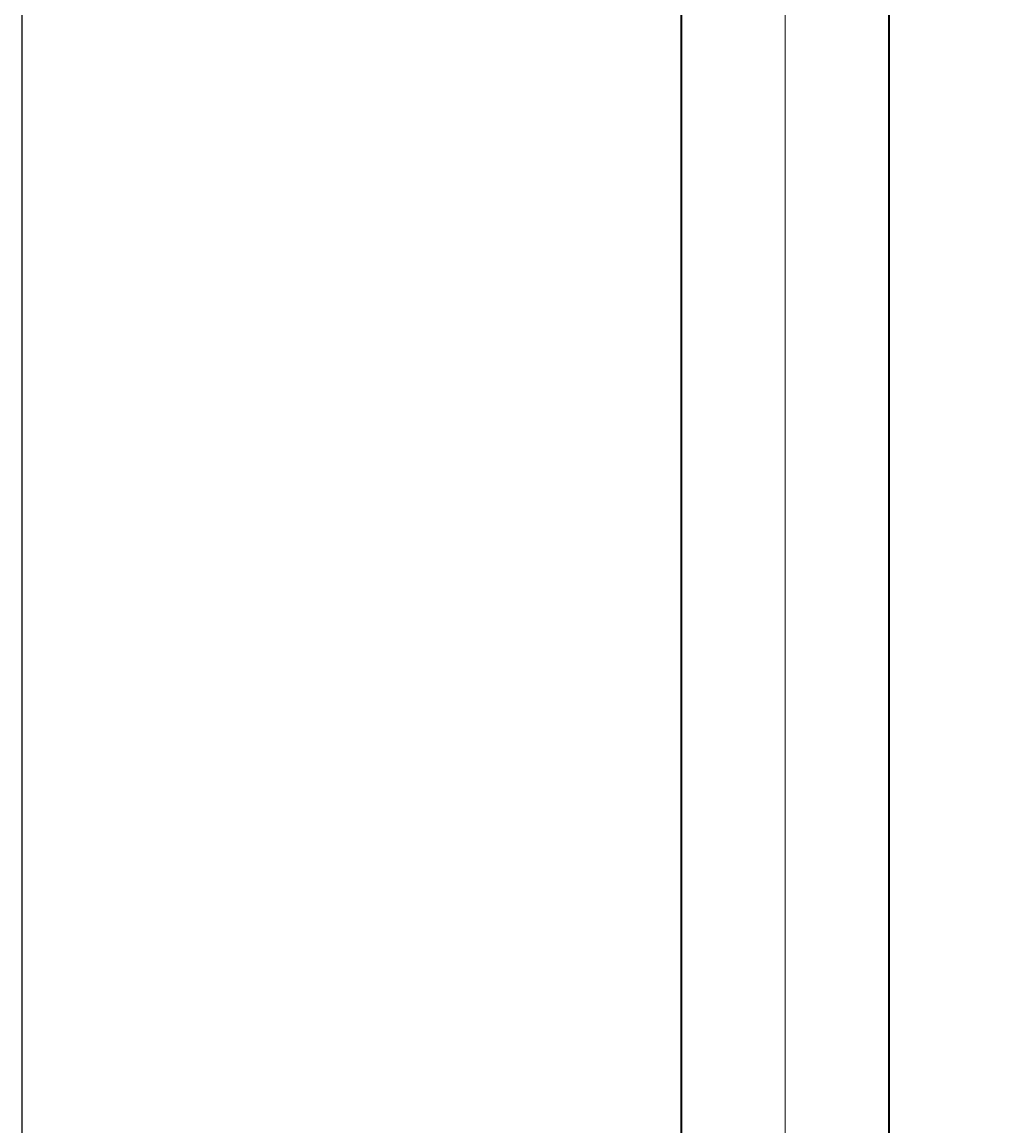
# Model space of a CAD drawing. Units: inches. Extents: x 1962 to 2771, y 1245 to 2660.
# Tile 44 of 114: x 2072 to 2093, y 2098 to 2122. Entities that reach past the tile are written whole.
import ezdxf

# ---------------------------------------------------------------- set-up
doc = ezdxf.new("R2010")
doc.units = ezdxf.units.IN
for name, color, linetype, lineweight in [('A-ANNO-DIMS', 2, 'Continuous', 18), ('A-GLAZ', 4, 'Continuous', 18), ('A-WALL', 7, 'Continuous', 35)]:
    doc.layers.add(name, color=color, linetype=linetype, lineweight=lineweight)
doc.styles.get("Standard").update_dxf_attribs({"font": 'arial.ttf'})
doc.dimstyles.get("Standard").update_dxf_attribs({"dimtxt": 0.18, "dimasz": 0.18, "dimexe": 0.18, "dimexo": 0.0625, "dimgap": 0.09, "dimtad": 0, "dimtih": 1, "dimtoh": 1, "dimdec": 4, "dimzin": 0, "dimdsep": 46, "dimtxsty": 'Standard', "dimcen": 0.09, "dimadec": 0, "dimazin": 0, "dimtfac": 1, "dimtdec": 4, "dimtofl": 0, "dimtmove": 0, "dimatfit": 3, "dimfxl": 1, "dimtolj": 1, "dimtzin": 0, "dimarcsym": 0})

# ---------------------------------------------------------------- blocks, each defined once
blk = doc.blocks.new('WIN-60IN-A')
blk.add_line((2.25, 60), (2.25, 0))
blk = doc.blocks.new('*D40')
at = {"layer": 'A-ANNO-DIMS', "color": 0, "lineweight": -2, "transparency": 16777216}
for p, q in [((2072.02, 2033.906), (2072.02, 2583.474)), ((2072.2, 2583.294), (2366.02, 2583.294)), ((2660.627, 2583.294), (2366.808, 2583.294)), ((2660.807, 2524.406), (2660.807, 2583.474))]:
    blk.add_line(p, q, dxfattribs=at)
at = {"layer": 'A-ANNO-DIMS', "color": 0, "transparency": 16777216}
for points in [[(2072.2, 2583.324), (2072.2, 2583.264), (2072.02, 2583.294)], [(2660.627, 2583.324), (2660.627, 2583.264), (2660.807, 2583.294)]]:
    blk.add_solid(points, dxfattribs=at)
at = {"layer": 'Defpoints', "color": 0, "transparency": 16777216}
for p in [(2660.807, 2583.294), (2660.807, 2524.344), (2072.02, 2033.844)]:
    blk.add_point(p, dxfattribs=at)
at = {"layer": 'A-ANNO-DIMS', "color": 0, "transparency": 16777216, "insert": (2366.414, 2583.294), "char_height": 0.18, "attachment_point": 5}
blk.add_mtext('\\A1;588.8', dxfattribs=at)
blk = doc.blocks.new('*D43')
at = {"layer": 'A-ANNO-DIMS', "color": 0, "lineweight": -2, "transparency": 16777216}
for p, q in [((2086.245, 2524.344), (2012.89, 2524.344)), ((2013.07, 2524.164), (2013.07, 2279.276)), ((2013.07, 2034.024), (2013.07, 2278.912)), ((2071.958, 2033.844), (2012.89, 2033.844))]:
    blk.add_line(p, q, dxfattribs=at)
at = {"layer": 'A-ANNO-DIMS', "color": 0, "transparency": 16777216}
for points in [[(2013.04, 2524.164), (2013.1, 2524.164), (2013.07, 2524.344)], [(2013.04, 2034.024), (2013.1, 2034.024), (2013.07, 2033.844)]]:
    blk.add_solid(points, dxfattribs=at)
at = {"layer": 'Defpoints', "color": 0, "transparency": 16777216}
for p in [(2086.307, 2524.344), (2013.07, 2033.844), (2072.02, 2033.844)]:
    blk.add_point(p, dxfattribs=at)
at = {"layer": 'A-ANNO-DIMS', "color": 0, "transparency": 16777216, "insert": (2013.07, 2279.094), "char_height": 0.18, "attachment_point": 5}
blk.add_mtext('\\A1;490.5', dxfattribs=at)

msp = doc.modelspace()

# ---------------------------------------------------------------- linework, layer by layer
at = {"layer": 'A-WALL'}
for p, q in [((2086.3074, 2471.8437), (2086.3074, 2033.8437)), ((2090.8074, 2177.8437), (2090.8074, 2033.8437))]:
    msp.add_line(p, q, dxfattribs=at)

# ---------------------------------------------------------------- block references
at = {"layer": 'A-GLAZ'}
msp.add_blockref('WIN-60IN-A', (2086.3074, 2080.0389), dxfattribs=at)

# ---------------------------------------------------------------- dimensions: what is measured, and where the dimension line sits
at = {"layer": 'A-ANNO-DIMS'}
dim = msp.add_linear_dim(base=(2660.8074, 2583.2937), p1=(2072.0204, 2033.8437), p2=(2660.8074, 2524.3437), dimstyle='Standard', override={"dimdec": 1, "dimlfac": 1, "dimrnd": 0, "dimzin": 0, "dimdsep": 46, "dimlunit": 2}, dxfattribs=at)
dim.commit()
dim.dimension.update_dxf_attribs({"geometry": '*D40', "text_midpoint": (2366.4139, 2583.2937)})
dim = msp.add_linear_dim(base=(2013.0704, 2033.8437), p1=(2086.3074, 2524.3437), p2=(2072.0204, 2033.8437), angle=90, dimstyle='Standard', override={"dimdec": 1, "dimlfac": 1, "dimrnd": 0, "dimzin": 0, "dimdsep": 46, "dimlunit": 2}, dxfattribs=at)
dim.commit()
dim.dimension.update_dxf_attribs({"geometry": '*D43', "text_midpoint": (2013.0704, 2279.0937)})

doc.saveas('drawing.dxf')
